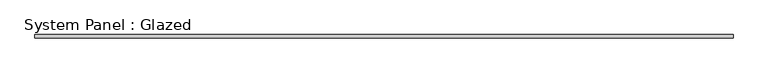
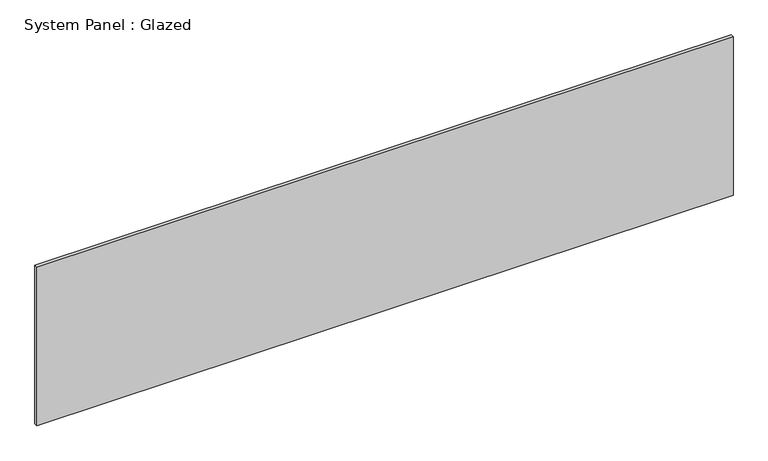
"""IFC4 building model written with IfcOpenShell, lengths in millimetres: plate geometry, System Panel : Glazed."""

from ifc_helpers import new_model, si_unit, origin, origin_with_axes, place, context, project, spatial, polyline, outline, extrude, source, transform, mapped, element, save


def system_panel_glazed_89838f9e(model_context):
    return source(origin(), model_context, "Body", "SweptSolid", [
        extrude(outline(polyline([(2536.4820739, 19.05), (-2536.4820739, 19.05), (-2536.4820739, 44.45), (2536.4820739, 44.45), (2536.4820739, 19.05)])), origin_with_axes(), (0.0, 0.0, 1.0), 1219.2),
    ])


if __name__ == "__main__":
    model = new_model("IFC4")
    model_context = context("Model", 3, world=origin())
    ifc_project = project(units=[si_unit("LENGTHUNIT", "METRE", prefix="MILLI")], contexts=[model_context])
    site = spatial("IfcSite", under=ifc_project)
    building = spatial("IfcBuilding", under=site)
    placement = place(None, origin())
    system_panel_glazed_shape = system_panel_glazed_89838f9e(model_context)
    element("IfcPlate", 1, ObjectType="System Panel : Glazed", at=placement, inside=building, context=model_context, shape_type="MappedRepresentation", body=[
        mapped(system_panel_glazed_shape, transform((0.0, 0.0, 0.0), x_axis=(1.0, 0.0, 0.0), y_axis=(0.0, 1.0, 0.0), z_axis=(0.0, 0.0, 1.0))),
    ])
    save(model, "model.ifc")

# Revit data of these elements
# Type "System Panel : Glazed"
#   Construction Type Id = "GSP4R"
#   Analytic Construction = "1/8 in Pilkington single glazing"
#   Visual Light Transmittance = 0.9
#   Solar Heat Gain Coefficient = 0.86
#   Heat Transfer Coefficient (U) = 1.18115 BTU/(h·ft²·°F)
# Element 1 (IfcPlate, "System Panel : Glazed")
#   Materials on its faces: "Glass"
# Materials
#   "Glass": class "Glass", colour RGB 0 128 192, transparency 0.75, Description = "Soda Lime Glass", Cost = 0
